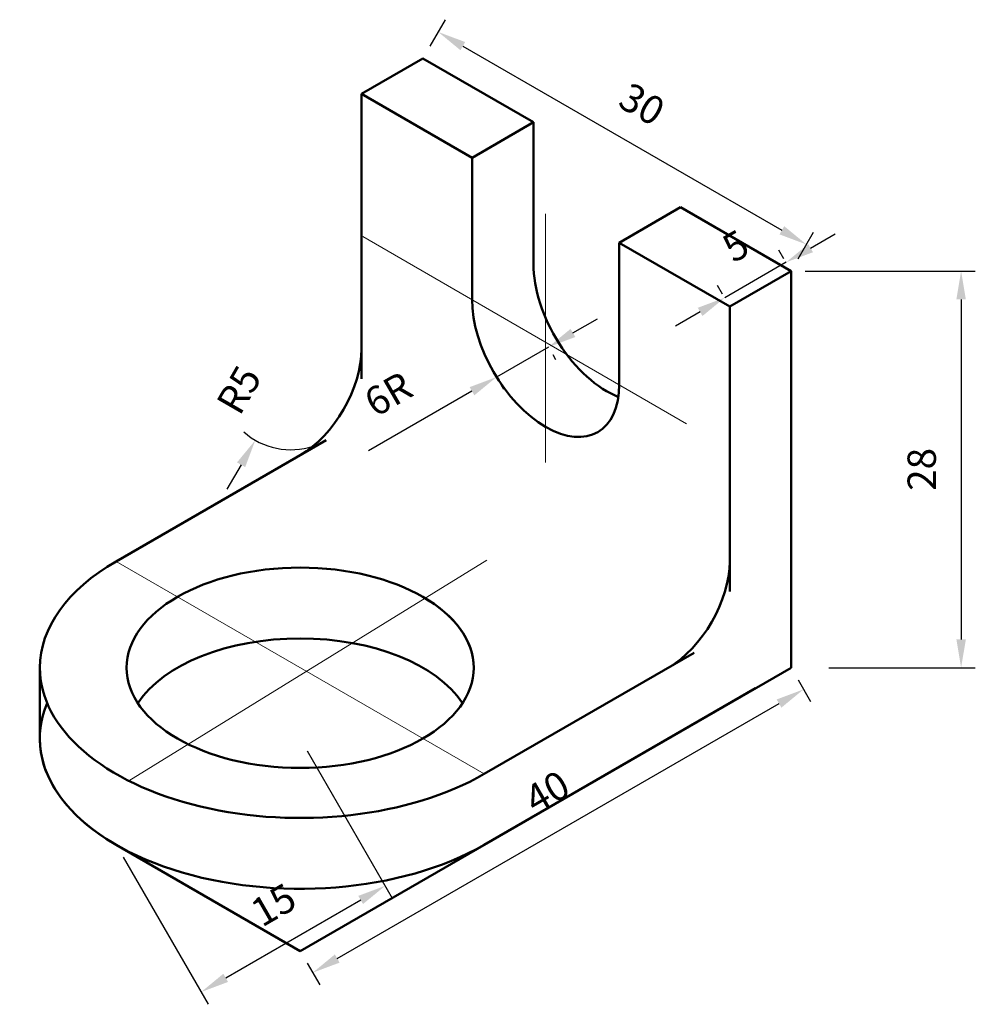
# Model space of a CAD drawing. Units: millimetres. Extents: x 2855.8 to 2923.2, y 1136.9 to 1206.4.
import ezdxf

# ---------------------------------------------------------------- set-up
doc = ezdxf.new("R2010")
doc.units = ezdxf.units.MM
doc.linetypes.add('CENTER', pattern=[50.8, 31.75, -6.35, 6.35, -6.35])
for name, color, linetype, lineweight in [('M-CNTR', 4, 'CENTER', 18), ('M-DIMS', 3, 'Continuous', 25), ('M-OUTL', 7, 'Continuous', 50)]:
    doc.layers.add(name, color=color, linetype=linetype, lineweight=lineweight)
doc.styles.get("Standard").update_dxf_attribs({"font": 'arial.ttf'})
doc.dimstyles.new('AM_ISO$0', dxfattribs={"dimtxt": 2, "dimasz": 2, "dimexe": 1, "dimexo": 1, "dimgap": 1.5, "dimtad": 1, "dimdsep": 46, "dimtxsty": 'Standard', "dimcen": 0, "dimclrd": 256, "dimclre": 256, "dimclrt": 2, "dimadec": 0, "dimazin": 2, "dimtp": 0.1, "dimtm": 0.1, "dimtfac": 0.71, "dimtmove": 0, "dimatfit": 3, "dimfxl": 1, "dimlwd": -1, "dimlwe": -1, "dimarcsym": 1})
doc.dimstyles.new('AM_ISO$4', dxfattribs={"dimtxt": 2, "dimasz": 2, "dimexe": 1, "dimexo": 1, "dimgap": 1.5, "dimtad": 1, "dimtoh": 1, "dimdsep": 46, "dimtxsty": 'Standard', "dimcen": 0, "dimclrd": 256, "dimclre": 256, "dimclrt": 2, "dimadec": 0, "dimazin": 2, "dimtp": 0.1, "dimtm": 0.1, "dimtfac": 0.71, "dimtofl": 0, "dimtmove": 0, "dimatfit": 0, "dimfxl": 1, "dimlwd": -1, "dimlwe": -1, "dimarcsym": 1})

# ---------------------------------------------------------------- blocks, each defined once
blk = doc.blocks.new('*D3')
at = {"layer": 'Defpoints', "color": 0, "transparency": 16777216}
for p in [(2910.206, 1188.685), (2911.873, 1160.685), (2922.206, 1160.685)]:
    blk.add_point(p, dxfattribs=at)
at = {"layer": 'M-DIMS', "color": 0, "linetype": 'ByBlock', "transparency": 16777216}
for p, q in [((2911.206, 1188.685), (2923.206, 1188.685)), ((2922.206, 1186.685), (2922.206, 1162.685)), ((2912.873, 1160.685), (2923.206, 1160.685))]:
    blk.add_line(p, q, dxfattribs=at)
at = {"layer": 'M-DIMS', "color": 0, "transparency": 16777216}
for points in [[(2921.873, 1186.685), (2922.54, 1186.685), (2922.206, 1188.685)], [(2921.873, 1162.685), (2922.54, 1162.685), (2922.206, 1160.685)]]:
    blk.add_solid(points, dxfattribs=at)
at = {"layer": 'M-DIMS', "color": 0, "transparency": 16777216, "insert": (2919.685, 1174.685), "char_height": 2, "attachment_point": 5, "rotation": 90}
blk.add_mtext('28', dxfattribs=at)
blk = doc.blocks.new('*D4')
at = {"layer": 'Defpoints', "color": 0, "transparency": 16777216}
for p in [(2910.206, 1160.685), (2911.088, 1159.157), (2875.565, 1140.685)]:
    blk.add_point(p, dxfattribs=at)
at = {"layer": 'M-DIMS', "color": 0, "linetype": 'ByBlock', "transparency": 16777216}
for p, q in [((2910.706, 1159.819), (2911.588, 1158.291)), ((2878.18, 1140.157), (2909.356, 1158.157)), ((2876.065, 1139.819), (2876.947, 1138.291))]:
    blk.add_line(p, q, dxfattribs=at)
at = {"layer": 'M-DIMS', "color": 0, "transparency": 16777216}
for points in [[(2909.19, 1158.446), (2909.523, 1157.868), (2911.088, 1159.157)], [(2878.013, 1140.446), (2878.346, 1139.868), (2876.447, 1139.157)]]:
    blk.add_solid(points, dxfattribs=at)
at = {"layer": 'M-DIMS', "color": 0, "transparency": 16777216, "insert": (2893.114, 1151.691), "char_height": 2, "attachment_point": 5, "rotation": 30}
blk.add_mtext('40', dxfattribs=at)
blk = doc.blocks.new('*D5')
at = {"layer": 'Defpoints', "color": 0, "transparency": 16777216}
for p in [(2910.206, 1188.685), (2905.52, 1186.801), (2905.876, 1186.185)]:
    blk.add_point(p, dxfattribs=at)
at = {"layer": 'M-DIMS', "color": 0, "linetype": 'ByBlock', "transparency": 16777216}
for p, q in [((2911.583, 1190.301), (2913.315, 1191.301)), ((2909.706, 1189.551), (2909.351, 1190.167)), ((2909.851, 1189.301), (2905.52, 1186.801)), ((2905.376, 1187.051), (2905.02, 1187.667)), ((2903.788, 1185.801), (2902.056, 1184.801))]:
    blk.add_line(p, q, dxfattribs=at)
at = {"layer": 'M-DIMS', "color": 0, "transparency": 16777216}
for points in [[(2911.416, 1190.59), (2911.749, 1190.012), (2909.851, 1189.301)], [(2903.622, 1186.09), (2903.955, 1185.512), (2905.52, 1186.801)]]:
    blk.add_solid(points, dxfattribs=at)
at = {"layer": 'M-DIMS', "color": 0, "transparency": 16777216, "insert": (2906.427, 1190.231), "char_height": 2, "attachment_point": 5, "rotation": 30}
blk.add_mtext('5', dxfattribs=at)
blk = doc.blocks.new('*D6')
at = {"layer": 'Defpoints', "color": 0, "transparency": 16777216}
for p in [(2875.565, 1155.685), (2862.575, 1148.185), (2881.565, 1145.292)]:
    blk.add_point(p, dxfattribs=at)
at = {"layer": 'M-DIMS', "color": 0, "linetype": 'ByBlock', "transparency": 16777216}
for p, q in [((2876.065, 1154.819), (2882.065, 1144.426)), ((2863.075, 1147.319), (2869.075, 1136.926)), ((2870.307, 1138.792), (2879.833, 1144.292))]:
    blk.add_line(p, q, dxfattribs=at)
at = {"layer": 'M-DIMS', "color": 0, "transparency": 16777216}
for points in [[(2879.667, 1144.581), (2880, 1144.004), (2881.565, 1145.292)], [(2870.14, 1139.081), (2870.474, 1138.504), (2868.575, 1137.792)]]:
    blk.add_solid(points, dxfattribs=at)
at = {"layer": 'M-DIMS', "color": 0, "transparency": 16777216, "insert": (2873.81, 1143.726), "char_height": 2, "attachment_point": 5, "rotation": 30}
blk.add_mtext('15', dxfattribs=at)
blk = doc.blocks.new('*D7')
at = {"layer": 'Defpoints', "color": 0, "transparency": 16777216}
for p in [(2884.226, 1203.685), (2911.289, 1190.56), (2910.206, 1188.685)]:
    blk.add_point(p, dxfattribs=at)
at = {"layer": 'M-DIMS', "color": 0, "linetype": 'ByBlock', "transparency": 16777216}
for p, q in [((2884.726, 1204.551), (2885.808, 1206.426)), ((2887.04, 1204.56), (2909.557, 1191.56)), ((2910.706, 1189.551), (2911.789, 1191.426))]:
    blk.add_line(p, q, dxfattribs=at)
at = {"layer": 'M-DIMS', "color": 0, "transparency": 16777216}
for points in [[(2887.207, 1204.849), (2886.874, 1204.271), (2885.308, 1205.56)], [(2909.724, 1191.849), (2909.39, 1191.271), (2911.289, 1190.56)]]:
    blk.add_solid(points, dxfattribs=at)
at = {"layer": 'M-DIMS', "color": 0, "transparency": 16777216, "insert": (2899.56, 1200.244), "char_height": 2, "attachment_point": 5, "rotation": 330}
blk.add_mtext('30', dxfattribs=at)
blk = doc.blocks.new('*D8')
at = {"layer": 'Defpoints', "color": 0, "transparency": 16777216}
for p in [(2874.896, 1181.071), (2872.396, 1176.741)]:
    blk.add_point(p, dxfattribs=at)
at = {"layer": 'M-DIMS', "color": 0, "linetype": 'ByBlock', "transparency": 16777216}
blk.add_line((2871.396, 1175.009), (2870.396, 1173.277), dxfattribs=at)
blk.add_arc((2874.896, 1181.071), 5, 228.54084, 288.54084, dxfattribs=at)
at = {"layer": 'M-DIMS', "color": 0, "transparency": 16777216}
blk.add_solid([(2871.107, 1175.176), (2871.684, 1174.843), (2872.396, 1176.741)], dxfattribs=at)
at = {"layer": 'M-DIMS', "color": 0, "transparency": 16777216, "insert": (2871.466, 1180.165), "char_height": 2, "attachment_point": 5, "rotation": 60}
blk.add_mtext('R5', dxfattribs=at)
blk = doc.blocks.new('*D9')
at = {"layer": 'Defpoints', "color": 0, "transparency": 16777216}
for p in [(2892.886, 1183.653), (2889.226, 1181.539), (2889.42, 1181.202)]:
    blk.add_point(p, dxfattribs=at)
at = {"layer": 'M-DIMS', "color": 0, "linetype": 'ByBlock', "transparency": 16777216}
for p, q in [((2894.813, 1184.316), (2896.545, 1185.316)), ((2893.081, 1183.316), (2889.42, 1181.202)), ((2893.386, 1182.787), (2893.581, 1182.45)), ((2887.688, 1180.202), (2880.387, 1175.987)), ((2889.726, 1180.673), (2889.92, 1180.336))]:
    blk.add_line(p, q, dxfattribs=at)
at = {"layer": 'M-DIMS', "color": 0, "transparency": 16777216}
for points in [[(2894.646, 1184.604), (2894.979, 1184.027), (2893.081, 1183.316)], [(2887.522, 1180.491), (2887.855, 1179.914), (2889.42, 1181.202)]]:
    blk.add_solid(points, dxfattribs=at)
at = {"layer": 'M-DIMS', "color": 0, "transparency": 16777216, "insert": (2881.911, 1179.778), "char_height": 2, "attachment_point": 5, "rotation": 30}
blk.add_mtext('6R', dxfattribs=at)

msp = doc.modelspace()

# ---------------------------------------------------------------- linework, layer by layer
at = {"layer": 'M-CNTR'}
for p, q in [((2892.886, 1183.685), (2892.886, 1192.718)), ((2892.886, 1192.718), (2892.886, 1175.172)), ((2879.994, 1191.128), (2902.817, 1177.894)), ((2862.575, 1168.185), (2888.556, 1153.185)), ((2888.727, 1168.284), (2863.465, 1152.704))]:
    msp.add_line(p, q, dxfattribs=at)
at = {"layer": 'M-OUTL'}
for p, q in [((2884.226, 1203.685), (2879.896, 1201.185)), ((2892.02, 1199.185), (2884.226, 1203.685)), ((2879.896, 1201.185), (2887.69, 1196.685)), ((2879.896, 1201.185), (2879.896, 1181.071)), ((2887.69, 1196.685), (2892.02, 1199.185)), ((2892.02, 1199.185), (2892.02, 1189.185)), ((2887.69, 1196.685), (2887.69, 1186.685)), ((2898.082, 1190.685), (2902.412, 1193.185)), ((2902.412, 1193.185), (2902.412, 1193.185)), ((2902.412, 1193.185), (2910.206, 1188.685)), ((2905.876, 1186.185), (2898.082, 1190.685)), ((2898.082, 1190.685), (2898.082, 1180.685)), ((2910.206, 1188.685), (2905.876, 1186.185)), ((2910.206, 1188.685), (2910.206, 1163.571)), ((2910.206, 1188.685), (2910.206, 1160.685)), ((2905.876, 1166.071), (2905.876, 1186.185)), ((2862.575, 1168.185), (2877.396, 1176.741)), ((2903.376, 1161.741), (2888.556, 1153.185)), ((2857.194, 1155.685), (2857.194, 1160.685)), ((2910.206, 1160.685), (2875.565, 1140.685)), ((2888.556, 1148.185), (2907.706, 1159.241)), ((2875.565, 1140.685), (2862.575, 1148.185))]:
    msp.add_line(p, q, dxfattribs=at)
for centre, major_axis, start_param, end_param in [((2897.216, 1186.185), (3.674, -6.364), 3.926991, 5.653048), ((2892.886, 1183.685), (3.674, -6.364), 3.926991, 7.068583), ((2875.565, 1180.685), (-3.062, -5.303), 0.785398, 2.356194), ((2875.565, 1160.685), (18.371, 0), 2.356194, 3.141593), ((2901.546, 1165.685), (-3.062, -5.303), 0.785398, 2.356194), ((2875.565, 1160.685), (12.247, 0), 0, 0.785398), ((2875.565, 1155.685), (-12.247, 0), 3.50296, 5.921818), ((2875.565, 1160.685), (18.371, 0), 3.141593, 5.497787), ((2875.565, 1155.685), (-18.371, 0), 6.045244, 8.63938), ((2875.565, 1155.685), (18.371, 0), 3.141593, 3.926991)]:
    msp.add_ellipse(centre, major_axis=major_axis, ratio=0.57735, start_param=start_param, end_param=end_param, dxfattribs=at)
msp.add_ellipse((2875.565, 1160.685), major_axis=(-12.247, 0), ratio=0.57735, dxfattribs=at)

# ---------------------------------------------------------------- dimensions: what is measured, and where the dimension line sits
at = {"layer": 'M-DIMS'}
for base, p1, p2, angle, picture, middle in [((2911.289, 1190.56), (2884.226, 1203.685), (2910.206, 1188.685), 330, '*D7', (2898.299, 1198.06)), ((2911.088, 1159.157), (2875.565, 1140.685), (2910.206, 1160.685), 30, '*D4', (2894.375, 1149.507))]:
    dim = msp.add_linear_dim(base=base, p1=p1, p2=p2, angle=angle, dimstyle='AM_ISO$0', override={"dimclrd": 0, "dimclre": 0, "dimclrt": 0}, dxfattribs=at)
    dim.commit()
    dim.dimension.update_dxf_attribs({"geometry": picture, "text_midpoint": middle, "dimtype": 161})
for p1, p2, distance, override, picture, middle in [((2910.206, 1188.685), (2905.876, 1186.185), -0.712, {"dimclrd": 0, "dimclre": 0, "dimclrt": 0}, '*D5', (2906.427, 1190.231)), ((2862.575, 1148.185), (2875.565, 1155.685), -12, {"dimpost": '', "dimclrd": 0, "dimclre": 0, "dimclrt": 0}, '*D6', (2873.81, 1143.726))]:
    dim = msp.add_aligned_dim(p1=p1, p2=p2, distance=distance, dimstyle='AM_ISO$0', override=override, dxfattribs=at)
    dim.commit()
    dim.dimension.update_dxf_attribs({"geometry": picture, "text_midpoint": middle})
dim = msp.add_linear_dim(base=(2922.206, 1160.685), p1=(2910.206, 1188.685), p2=(2911.873, 1160.685), angle=90, dimstyle='AM_ISO$0', override={"dimpost": '', "dimclrd": 0, "dimclre": 0, "dimclrt": 0}, dxfattribs=at)
dim.commit()
dim.dimension.update_dxf_attribs({"geometry": '*D3', "text_midpoint": (2919.685, 1174.685)})
dim = msp.add_aligned_dim(p1=(2892.886, 1183.653), p2=(2889.226, 1181.539), distance=0.389, text='6R', dimstyle='AM_ISO$0', override={"dimpost": '', "dimclrd": 0, "dimclre": 0, "dimclrt": 0}, dxfattribs=at)
dim.commit()
dim.dimension.update_dxf_attribs({"geometry": '*D9', "text_midpoint": (2881.911, 1179.778)})
dim = msp.add_radius_dim(center=(2874.896, 1181.071), mpoint=(2872.396, 1176.741), dimstyle='AM_ISO$4', override={"dimpost": '', "dimclrd": 0, "dimclre": 0, "dimclrt": 0}, dxfattribs=at)
dim.commit()
dim.dimension.update_dxf_attribs({"geometry": '*D8', "text_midpoint": (2873.646, 1178.906), "dimtype": 164})

doc.saveas('drawing.dxf')
